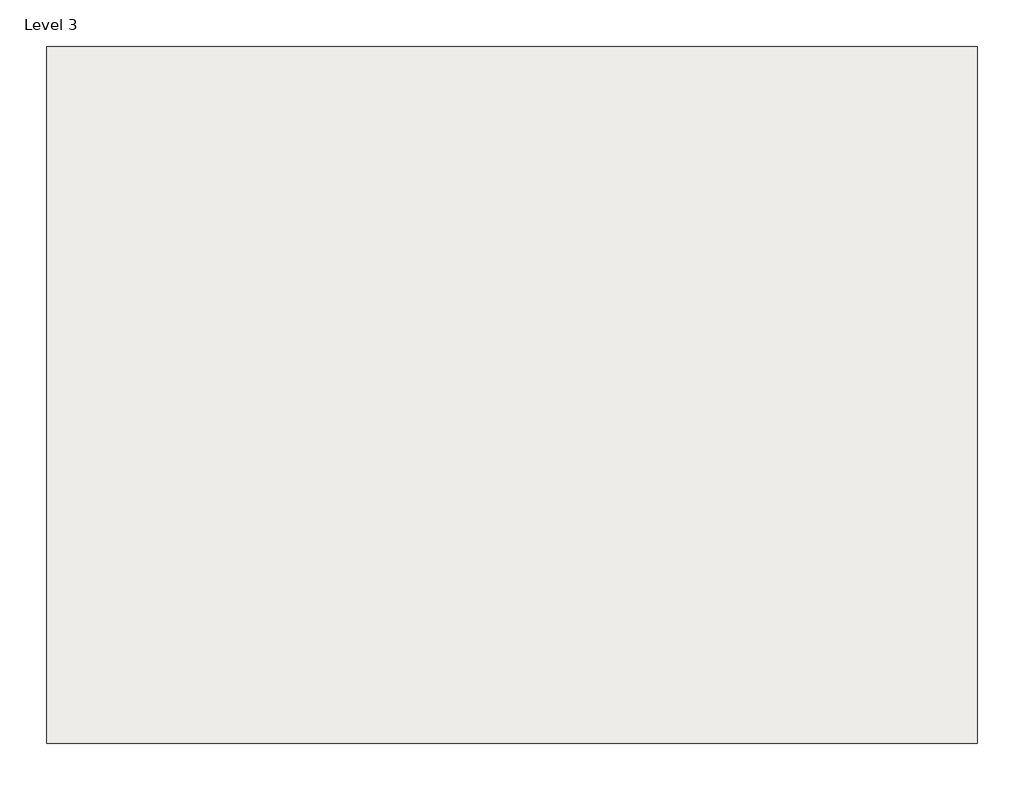
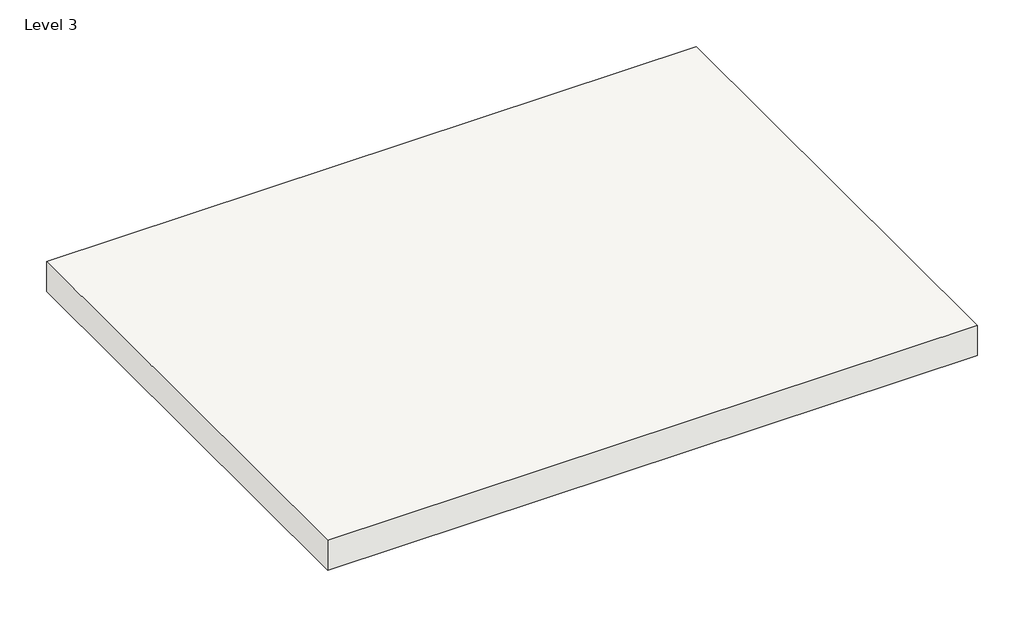
# One storey: 1 slab.
"""IFC4 building model written with IfcOpenShell, lengths in millimetres."""

from ifc_helpers import new_model, si_unit, frame, origin, place, context, project, spatial, polyline, outline, extrude, element, save

model = new_model("IFC4")

# Units and contexts
model_context = context("Model", 3, world=origin())
ifc_project = project(units=[si_unit("LENGTHUNIT", "METRE", prefix="MILLI")], contexts=[model_context])

# Site, building, storey
site = spatial("IfcSite", under=ifc_project)
building = spatial("IfcBuilding", under=site)
storey = spatial("IfcBuildingStorey", under=building, Name="Level 3", Elevation=9144.0)

# Slab
placement = place(None, origin())
element("IfcSlab", 1, ObjectType="Generic Floor - 400mm", at=placement, inside=storey, context=model_context, shape_type="SweptSolid", body=[
    extrude(outline(polyline([(11861.7023789, 3004.8489075), (11861.7023789, -3138.7510925), (3660.4261575, -3138.7510925), (3660.4261575, 3004.8489075), (11861.7023789, 3004.8489075)])), frame((0.0, 0.0, 8744.0), z_axis=(0.0, 0.0, 1.0), x_axis=(1.0, 0.0, 0.0)), (0.0, 0.0, 1.0), 400.0),
])

save(model, "model.ifc")

# Revit data of these elements
# Type "Generic Floor - 400mm"
#   Function = 0
#   Layers, outside or top first: 1' - 3.74803" no material (function 1)
# Element 1 (IfcSlab, "Generic Floor - 400mm")
#   Height Offset From Level = 0' - 0"
#   Phase Created = New Construction
#   Materials on its faces: "Default Roof"
# Materials
#   "Default Roof": colour RGB 80 80 80, transparency 0
